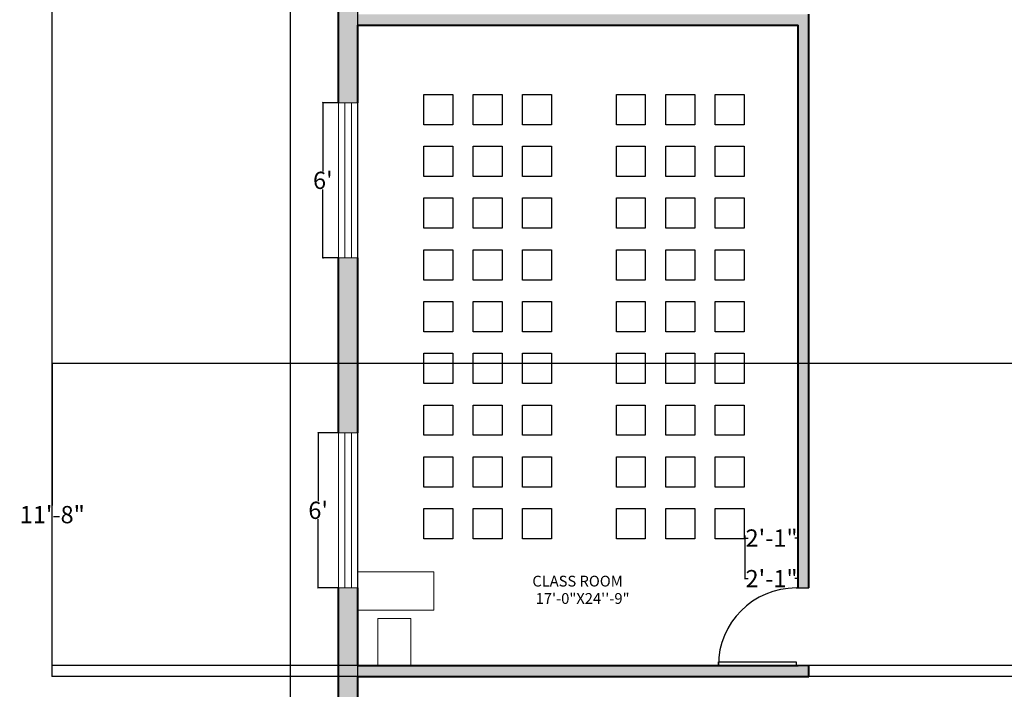
# Model space of a CAD drawing. Units: inches. Extents: x -405 to 940, y 226 to 2032.
# Tile 3 of 10: x -405 to 51, y 846 to 1156. Entities that reach past the tile are written whole.
import ezdxf

# ---------------------------------------------------------------- set-up
doc = ezdxf.new("R2010")
doc.units = ezdxf.units.IN
doc.header["$MEASUREMENT"] = 0
doc.linetypes.add('ACAD_ISO02W100', pattern=[15, 12, -3])
for name, color, linetype, lineweight in [('A-ANNO-DIMS', 120, 'Continuous', 18), ('A-AREA-IDEN', 32, 'Continuous', 18), ('A-FURN-SEAT', 5, 'Continuous', 18), ('A-GLAZ-HIDN', 1, 'ACAD_ISO02W100', 18), ('A-WALL-PATT', 8, 'Continuous', 13), ('door', 6, 'Continuous', 25), ('tables', 2, 'Continuous', 18), ('wall', 3, 'Continuous', 40), ('window', 1, 'Continuous', 18)]:
    doc.layers.add(name, color=color, linetype=linetype, lineweight=lineweight)
doc.layers.add('beches', color=5, linetype='Continuous')
doc.styles.get("Standard").update_dxf_attribs({"font": 'arial.ttf'})
doc.dimstyles.get("Standard").update_dxf_attribs({"dimtxt": 8, "dimasz": 0.18, "dimexe": 0.18, "dimexo": 0.0625, "dimgap": 0.09, "dimtad": 0, "dimtih": 1, "dimtoh": 1, "dimdec": 0, "dimzin": 0, "dimdsep": 46, "dimlunit": 3, "dimtxsty": 'Standard', "dimblk": 'OBLIQUE', "dimcen": 0.09, "dimadec": 0, "dimazin": 0, "dimtfac": 1, "dimtdec": 0, "dimtofl": 0, "dimtmove": 0, "dimatfit": 3, "dimfxl": 1, "dimtolj": 1, "dimtzin": 0, "dimarcsym": 0})

# ---------------------------------------------------------------- blocks, each defined once
blk = doc.blocks.new('*U4')
for p, q in [((0, 0), (0, -6)), ((36, 0), (36, -6))]:
    blk.add_line(p, q)
blk.add_lwpolyline([(0, 0), (0, 36), (1.75, 36), (1.75, 0)], close=True)
blk.add_arc((0, 0), 36, 0, 90)
blk = doc.blocks.new('*U13')
at = {"layer": 'beches'}
blk.add_lwpolyline([(6.71, -7.02), (-6.71, -7.02), (-6.71, 7.02), (6.71, 7.02)], close=True, dxfattribs=at)
blk = doc.blocks.new('*U14')
at = {"layer": 'A-FURN-SEAT', "transparency": 16777216}
for p in [(-45.84, 192), (-45.84, 192, 12), (-45.84, 192, 24), (-45.84, 192, 36), (-45.84, 192, 48), (-45.84, 192, 60), (-45.84, 192, 72), (-45.84, 192, 84), (-45.84, 192, 96), (-45.84, 192, 108), (-45.84, 192, 120), (-45.84, 192, 132), (-22.92, 192), (-22.92, 192, 12), (-22.92, 192, 24), (-22.92, 192, 36), (-22.92, 192, 48), (-22.92, 192, 60), (-22.92, 192, 72), (-22.92, 192, 84), (-22.92, 192, 96), (-22.92, 192, 108), (-22.92, 192, 120), (-22.92, 192, 132), (0, 192), (0, 192, 12), (0, 192, 24), (0, 192, 36), (0, 192, 48), (0, 192, 60), (0, 192, 72), (0, 192, 84), (0, 192, 96), (0, 192, 108), (0, 192, 120), (0, 192, 132), (-45.84, 168), (-45.84, 168, 12), (-45.84, 168, 24), (-45.84, 168, 36), (-45.84, 168, 48), (-45.84, 168, 60), (-45.84, 168, 72), (-45.84, 168, 84), (-45.84, 168, 96), (-45.84, 168, 108), (-45.84, 168, 120), (-45.84, 168, 132), (-22.92, 168), (-22.92, 168, 12), (-22.92, 168, 24), (-22.92, 168, 36), (-22.92, 168, 48), (-22.92, 168, 60), (-22.92, 168, 72), (-22.92, 168, 84), (-22.92, 168, 96), (-22.92, 168, 108), (-22.92, 168, 120), (-22.92, 168, 132), (0, 168), (0, 168, 12), (0, 168, 24), (0, 168, 36), (0, 168, 48), (0, 168, 60), (0, 168, 72), (0, 168, 84), (0, 168, 96), (0, 168, 108), (0, 168, 120), (0, 168, 132), (-45.84, 144), (-45.84, 144, 12), (-45.84, 144, 24), (-45.84, 144, 36), (-45.84, 144, 48), (-45.84, 144, 60), (-45.84, 144, 72), (-45.84, 144, 84), (-45.84, 144, 96), (-45.84, 144, 108), (-45.84, 144, 120), (-45.84, 144, 132), (-22.92, 144), (-22.92, 144, 12), (-22.92, 144, 24), (-22.92, 144, 36), (-22.92, 144, 48), (-22.92, 144, 60), (-22.92, 144, 72), (-22.92, 144, 84), (-22.92, 144, 96), (-22.92, 144, 108), (-22.92, 144, 120), (-22.92, 144, 132), (0, 144), (0, 144, 12), (0, 144, 24), (0, 144, 36), (0, 144, 48), (0, 144, 60), (0, 144, 72), (0, 144, 84), (0, 144, 96), (0, 144, 108), (0, 144, 120), (0, 144, 132), (-45.84, 120), (-45.84, 120, 12), (-45.84, 120, 24), (-45.84, 120, 36), (-45.84, 120, 48), (-45.84, 120, 60), (-45.84, 120, 72), (-45.84, 120, 84), (-45.84, 120, 96), (-45.84, 120, 108), (-45.84, 120, 120), (-45.84, 120, 132), (-22.92, 120), (-22.92, 120, 12), (-22.92, 120, 24), (-22.92, 120, 36), (-22.92, 120, 48), (-22.92, 120, 60), (-22.92, 120, 72), (-22.92, 120, 84), (-22.92, 120, 96), (-22.92, 120, 108), (-22.92, 120, 120), (-22.92, 120, 132), (0, 120), (0, 120, 12), (0, 120, 24), (0, 120, 36), (0, 120, 48), (0, 120, 60), (0, 120, 72), (0, 120, 84), (0, 120, 96), (0, 120, 108), (0, 120, 120), (0, 120, 132), (-45.84, 96), (-45.84, 96, 12), (-45.84, 96, 24), (-45.84, 96, 36), (-45.84, 96, 48), (-45.84, 96, 60), (-45.84, 96, 72), (-45.84, 96, 84), (-45.84, 96, 96), (-45.84, 96, 108), (-45.84, 96, 120), (-45.84, 96, 132), (-22.92, 96), (-22.92, 96, 12), (-22.92, 96, 24), (-22.92, 96, 36), (-22.92, 96, 48), (-22.92, 96, 60), (-22.92, 96, 72), (-22.92, 96, 84), (-22.92, 96, 96), (-22.92, 96, 108), (-22.92, 96, 120), (-22.92, 96, 132), (0, 96), (0, 96, 12), (0, 96, 24), (0, 96, 36), (0, 96, 48), (0, 96, 60), (0, 96, 72), (0, 96, 84), (0, 96, 96), (0, 96, 108), (0, 96, 120), (0, 96, 132), (-45.84, 72), (-45.84, 72, 12), (-45.84, 72, 24), (-45.84, 72, 36), (-45.84, 72, 48), (-45.84, 72, 60), (-45.84, 72, 72), (-45.84, 72, 84), (-45.84, 72, 96), (-45.84, 72, 108), (-45.84, 72, 120), (-45.84, 72, 132), (-22.92, 72), (-22.92, 72, 12), (-22.92, 72, 24), (-22.92, 72, 36), (-22.92, 72, 48), (-22.92, 72, 60), (-22.92, 72, 72), (-22.92, 72, 84), (-22.92, 72, 96), (-22.92, 72, 108), (-22.92, 72, 120), (-22.92, 72, 132), (0, 72), (0, 72, 12), (0, 72, 24), (0, 72, 36), (0, 72, 48), (0, 72, 60), (0, 72, 72), (0, 72, 84), (0, 72, 96), (0, 72, 108), (0, 72, 120), (0, 72, 132), (-45.84, 48), (-45.84, 48, 12), (-45.84, 48, 24), (-45.84, 48, 36), (-45.84, 48, 48), (-45.84, 48, 60), (-45.84, 48, 72), (-45.84, 48, 84), (-45.84, 48, 96), (-45.84, 48, 108), (-45.84, 48, 120), (-45.84, 48, 132), (-22.92, 48), (-22.92, 48, 12), (-22.92, 48, 24), (-22.92, 48, 36), (-22.92, 48, 48), (-22.92, 48, 60), (-22.92, 48, 72), (-22.92, 48, 84), (-22.92, 48, 96), (-22.92, 48, 108), (-22.92, 48, 120), (-22.92, 48, 132), (0, 48), (0, 48, 12), (0, 48, 24), (0, 48, 36), (0, 48, 48), (0, 48, 60), (0, 48, 72), (0, 48, 84), (0, 48, 96), (0, 48, 108), (0, 48, 120), (0, 48, 132), (-45.84, 24), (-45.84, 24, 12), (-45.84, 24, 24), (-45.84, 24, 36), (-45.84, 24, 48), (-45.84, 24, 60), (-45.84, 24, 72), (-45.84, 24, 84), (-45.84, 24, 96), (-45.84, 24, 108), (-45.84, 24, 120), (-45.84, 24, 132), (-22.92, 24), (-22.92, 24, 12), (-22.92, 24, 24), (-22.92, 24, 36), (-22.92, 24, 48), (-22.92, 24, 60), (-22.92, 24, 72), (-22.92, 24, 84), (-22.92, 24, 96), (-22.92, 24, 108), (-22.92, 24, 120), (-22.92, 24, 132), (0, 24), (0, 24, 12), (0, 24, 24), (0, 24, 36), (0, 24, 48), (0, 24, 60), (0, 24, 72), (0, 24, 84), (0, 24, 96), (0, 24, 108), (0, 24, 120), (0, 24, 132), (-45.84, 0), (-45.84, 0, 12), (-45.84, 0, 24), (-45.84, 0, 36), (-45.84, 0, 48), (-45.84, 0, 60), (-45.84, 0, 72), (-45.84, 0, 84), (-45.84, 0, 96), (-45.84, 0, 108), (-45.84, 0, 120), (-45.84, 0, 132), (-22.92, 0), (-22.92, 0, 12), (-22.92, 0, 24), (-22.92, 0, 36), (-22.92, 0, 48), (-22.92, 0, 60), (-22.92, 0, 72), (-22.92, 0, 84), (-22.92, 0, 96), (-22.92, 0, 108), (-22.92, 0, 120), (-22.92, 0, 132), (0, 0), (0, 0, 12), (0, 0, 24), (0, 0, 36), (0, 0, 48), (0, 0, 60), (0, 0, 72), (0, 0, 84), (0, 0, 96), (0, 0, 108), (0, 0, 120), (0, 0, 132)]:
    blk.add_blockref('*U13', p, dxfattribs=at)
blk = doc.blocks.new('*U11')
at = {"layer": 'beches'}
blk.add_lwpolyline([(6.71, -7.02), (-6.71, -7.02), (-6.71, 7.02), (6.71, 7.02)], close=True, dxfattribs=at)
blk = doc.blocks.new('*U12')
at = {"layer": 'A-FURN-SEAT', "transparency": 16777216}
for p in [(-45.84, 192), (-45.84, 192, 12), (-45.84, 192, 24), (-45.84, 192, 36), (-45.84, 192, 48), (-45.84, 192, 60), (-45.84, 192, 72), (-45.84, 192, 84), (-45.84, 192, 96), (-45.84, 192, 108), (-45.84, 192, 120), (-45.84, 192, 132), (-22.92, 192), (-22.92, 192, 12), (-22.92, 192, 24), (-22.92, 192, 36), (-22.92, 192, 48), (-22.92, 192, 60), (-22.92, 192, 72), (-22.92, 192, 84), (-22.92, 192, 96), (-22.92, 192, 108), (-22.92, 192, 120), (-22.92, 192, 132), (0, 192), (0, 192, 12), (0, 192, 24), (0, 192, 36), (0, 192, 48), (0, 192, 60), (0, 192, 72), (0, 192, 84), (0, 192, 96), (0, 192, 108), (0, 192, 120), (0, 192, 132), (-45.84, 168), (-45.84, 168, 12), (-45.84, 168, 24), (-45.84, 168, 36), (-45.84, 168, 48), (-45.84, 168, 60), (-45.84, 168, 72), (-45.84, 168, 84), (-45.84, 168, 96), (-45.84, 168, 108), (-45.84, 168, 120), (-45.84, 168, 132), (-22.92, 168), (-22.92, 168, 12), (-22.92, 168, 24), (-22.92, 168, 36), (-22.92, 168, 48), (-22.92, 168, 60), (-22.92, 168, 72), (-22.92, 168, 84), (-22.92, 168, 96), (-22.92, 168, 108), (-22.92, 168, 120), (-22.92, 168, 132), (0, 168), (0, 168, 12), (0, 168, 24), (0, 168, 36), (0, 168, 48), (0, 168, 60), (0, 168, 72), (0, 168, 84), (0, 168, 96), (0, 168, 108), (0, 168, 120), (0, 168, 132), (-45.84, 144), (-45.84, 144, 12), (-45.84, 144, 24), (-45.84, 144, 36), (-45.84, 144, 48), (-45.84, 144, 60), (-45.84, 144, 72), (-45.84, 144, 84), (-45.84, 144, 96), (-45.84, 144, 108), (-45.84, 144, 120), (-45.84, 144, 132), (-22.92, 144), (-22.92, 144, 12), (-22.92, 144, 24), (-22.92, 144, 36), (-22.92, 144, 48), (-22.92, 144, 60), (-22.92, 144, 72), (-22.92, 144, 84), (-22.92, 144, 96), (-22.92, 144, 108), (-22.92, 144, 120), (-22.92, 144, 132), (0, 144), (0, 144, 12), (0, 144, 24), (0, 144, 36), (0, 144, 48), (0, 144, 60), (0, 144, 72), (0, 144, 84), (0, 144, 96), (0, 144, 108), (0, 144, 120), (0, 144, 132), (-45.84, 120), (-45.84, 120, 12), (-45.84, 120, 24), (-45.84, 120, 36), (-45.84, 120, 48), (-45.84, 120, 60), (-45.84, 120, 72), (-45.84, 120, 84), (-45.84, 120, 96), (-45.84, 120, 108), (-45.84, 120, 120), (-45.84, 120, 132), (-22.92, 120), (-22.92, 120, 12), (-22.92, 120, 24), (-22.92, 120, 36), (-22.92, 120, 48), (-22.92, 120, 60), (-22.92, 120, 72), (-22.92, 120, 84), (-22.92, 120, 96), (-22.92, 120, 108), (-22.92, 120, 120), (-22.92, 120, 132), (0, 120), (0, 120, 12), (0, 120, 24), (0, 120, 36), (0, 120, 48), (0, 120, 60), (0, 120, 72), (0, 120, 84), (0, 120, 96), (0, 120, 108), (0, 120, 120), (0, 120, 132), (-45.84, 96), (-45.84, 96, 12), (-45.84, 96, 24), (-45.84, 96, 36), (-45.84, 96, 48), (-45.84, 96, 60), (-45.84, 96, 72), (-45.84, 96, 84), (-45.84, 96, 96), (-45.84, 96, 108), (-45.84, 96, 120), (-45.84, 96, 132), (-22.92, 96), (-22.92, 96, 12), (-22.92, 96, 24), (-22.92, 96, 36), (-22.92, 96, 48), (-22.92, 96, 60), (-22.92, 96, 72), (-22.92, 96, 84), (-22.92, 96, 96), (-22.92, 96, 108), (-22.92, 96, 120), (-22.92, 96, 132), (0, 96), (0, 96, 12), (0, 96, 24), (0, 96, 36), (0, 96, 48), (0, 96, 60), (0, 96, 72), (0, 96, 84), (0, 96, 96), (0, 96, 108), (0, 96, 120), (0, 96, 132), (-45.84, 72), (-45.84, 72, 12), (-45.84, 72, 24), (-45.84, 72, 36), (-45.84, 72, 48), (-45.84, 72, 60), (-45.84, 72, 72), (-45.84, 72, 84), (-45.84, 72, 96), (-45.84, 72, 108), (-45.84, 72, 120), (-45.84, 72, 132), (-22.92, 72), (-22.92, 72, 12), (-22.92, 72, 24), (-22.92, 72, 36), (-22.92, 72, 48), (-22.92, 72, 60), (-22.92, 72, 72), (-22.92, 72, 84), (-22.92, 72, 96), (-22.92, 72, 108), (-22.92, 72, 120), (-22.92, 72, 132), (0, 72), (0, 72, 12), (0, 72, 24), (0, 72, 36), (0, 72, 48), (0, 72, 60), (0, 72, 72), (0, 72, 84), (0, 72, 96), (0, 72, 108), (0, 72, 120), (0, 72, 132), (-45.84, 48), (-45.84, 48, 12), (-45.84, 48, 24), (-45.84, 48, 36), (-45.84, 48, 48), (-45.84, 48, 60), (-45.84, 48, 72), (-45.84, 48, 84), (-45.84, 48, 96), (-45.84, 48, 108), (-45.84, 48, 120), (-45.84, 48, 132), (-22.92, 48), (-22.92, 48, 12), (-22.92, 48, 24), (-22.92, 48, 36), (-22.92, 48, 48), (-22.92, 48, 60), (-22.92, 48, 72), (-22.92, 48, 84), (-22.92, 48, 96), (-22.92, 48, 108), (-22.92, 48, 120), (-22.92, 48, 132), (0, 48), (0, 48, 12), (0, 48, 24), (0, 48, 36), (0, 48, 48), (0, 48, 60), (0, 48, 72), (0, 48, 84), (0, 48, 96), (0, 48, 108), (0, 48, 120), (0, 48, 132), (-45.84, 24), (-45.84, 24, 12), (-45.84, 24, 24), (-45.84, 24, 36), (-45.84, 24, 48), (-45.84, 24, 60), (-45.84, 24, 72), (-45.84, 24, 84), (-45.84, 24, 96), (-45.84, 24, 108), (-45.84, 24, 120), (-45.84, 24, 132), (-22.92, 24), (-22.92, 24, 12), (-22.92, 24, 24), (-22.92, 24, 36), (-22.92, 24, 48), (-22.92, 24, 60), (-22.92, 24, 72), (-22.92, 24, 84), (-22.92, 24, 96), (-22.92, 24, 108), (-22.92, 24, 120), (-22.92, 24, 132), (0, 24), (0, 24, 12), (0, 24, 24), (0, 24, 36), (0, 24, 48), (0, 24, 60), (0, 24, 72), (0, 24, 84), (0, 24, 96), (0, 24, 108), (0, 24, 120), (0, 24, 132), (-45.84, 0), (-45.84, 0, 12), (-45.84, 0, 24), (-45.84, 0, 36), (-45.84, 0, 48), (-45.84, 0, 60), (-45.84, 0, 72), (-45.84, 0, 84), (-45.84, 0, 96), (-45.84, 0, 108), (-45.84, 0, 120), (-45.84, 0, 132), (-22.92, 0), (-22.92, 0, 12), (-22.92, 0, 24), (-22.92, 0, 36), (-22.92, 0, 48), (-22.92, 0, 60), (-22.92, 0, 72), (-22.92, 0, 84), (-22.92, 0, 96), (-22.92, 0, 108), (-22.92, 0, 120), (-22.92, 0, 132), (0, 0), (0, 0, 12), (0, 0, 24), (0, 0, 36), (0, 0, 48), (0, 0, 60), (0, 0, 72), (0, 0, 84), (0, 0, 96), (0, 0, 108), (0, 0, 120), (0, 0, 132)]:
    blk.add_blockref('*U11', p, dxfattribs=at)
blk = doc.blocks.new('_Oblique')
at = {"color": 0, "linetype": 'ByBlock', "lineweight": -2}
blk.add_line((-0.5, -0.5), (0.5, 0.5), dxfattribs=at)
blk = doc.blocks.new('*D44')
at = {"layer": 'A-ANNO-DIMS', "color": 0, "lineweight": -2, "transparency": 16777216}
for p, q in [((-257.29, 1887.81), (-279.61, 1887.81)), ((-279.43, 1887.81), (-279.43, 1210.99)), ((-279.43, 525.81), (-279.43, 1202.63)), ((-257.29, 525.81), (-279.61, 525.81))]:
    blk.add_line(p, q, dxfattribs=at)
at = {"layer": 'Defpoints', "color": 0, "transparency": 16777216}
for p in [(-257.23, 1887.81), (-279.43, 525.81), (-257.23, 525.81)]:
    blk.add_point(p, dxfattribs=at)
at = {"layer": 'A-ANNO-DIMS', "color": 0, "lineweight": -2, "transparency": 16777216, "xscale": 0.18, "yscale": 0.18, "zscale": 0.18}
for p, rotation in [((-279.43, 1887.81), 90), ((-279.43, 525.81), 270)]:
    blk.add_blockref('_Oblique', p, dxfattribs=dict(at, rotation=rotation))
at = {"layer": 'A-ANNO-DIMS', "color": 0, "transparency": 16777216, "insert": (-279.43, 1206.81), "char_height": 8, "attachment_point": 5}
blk.add_mtext('\\A1;113\'-6"', dxfattribs=at)
blk = doc.blocks.new('*D45')
at = {"layer": 'A-ANNO-DIMS', "color": 0, "lineweight": -2, "transparency": 16777216}
for p, q in [((-68.93, 917.09), (-68.93, 915.78)), ((-44.23, 917.09), (-44.23, 915.78)), ((-68.93, 915.96), (-67.37, 915.96)), ((-44.23, 915.96), (-45.79, 915.96))]:
    blk.add_line(p, q, dxfattribs=at)
at = {"layer": 'Defpoints', "color": 0, "transparency": 16777216}
for p in [(-68.93, 917.16), (-44.23, 917.16), (-68.93, 915.96)]:
    blk.add_point(p, dxfattribs=at)
at = {"layer": 'A-ANNO-DIMS', "color": 0, "lineweight": -2, "transparency": 16777216, "xscale": 0.18, "yscale": 0.18, "zscale": 0.18, "rotation": 180}
blk.add_blockref('_Oblique', (-68.93, 915.96), dxfattribs=at)
at = {"layer": 'A-ANNO-DIMS', "color": 0, "lineweight": -2, "transparency": 16777216, "xscale": 0.18, "yscale": 0.18, "zscale": 0.18}
blk.add_blockref('_Oblique', (-44.23, 915.96), dxfattribs=at)
at = {"layer": 'A-ANNO-DIMS', "color": 0, "transparency": 16777216, "insert": (-56.58, 915.96), "char_height": 8, "attachment_point": 5}
blk.add_mtext('\\A1;2\'-1"', dxfattribs=at)
blk = doc.blocks.new('*D46')
at = {"layer": 'A-ANNO-DIMS', "color": 0, "lineweight": -2, "transparency": 16777216}
for p, q in [((-68.93, 915.72), (-68.93, 896.95)), ((-68.93, 897.13), (-67.37, 897.13)), ((-44.23, 897.13), (-45.79, 897.13)), ((-44.23, 892.87), (-44.23, 897.31))]:
    blk.add_line(p, q, dxfattribs=at)
at = {"layer": 'Defpoints', "color": 0, "transparency": 16777216}
for p in [(-68.93, 915.78), (-44.23, 897.13), (-44.23, 892.81)]:
    blk.add_point(p, dxfattribs=at)
at = {"layer": 'A-ANNO-DIMS', "color": 0, "lineweight": -2, "transparency": 16777216, "xscale": 0.18, "yscale": 0.18, "zscale": 0.18, "rotation": 180}
blk.add_blockref('_Oblique', (-68.93, 897.13), dxfattribs=at)
at = {"layer": 'A-ANNO-DIMS', "color": 0, "lineweight": -2, "transparency": 16777216, "xscale": 0.18, "yscale": 0.18, "zscale": 0.18}
blk.add_blockref('_Oblique', (-44.23, 897.13), dxfattribs=at)
at = {"layer": 'A-ANNO-DIMS', "color": 0, "transparency": 16777216, "insert": (-56.58, 897.13), "char_height": 8, "attachment_point": 5}
blk.add_mtext('\\A1;2\'-1"', dxfattribs=at)
blk = doc.blocks.new('*D53')
at = {"layer": 'A-ANNO-DIMS', "color": 0, "lineweight": -2, "transparency": 16777216}
for p, q in [((-257.29, 964.81), (-266.86, 964.81)), ((-266.68, 964.81), (-266.68, 932.98)), ((-266.68, 892.81), (-266.68, 924.64)), ((-257.29, 892.81), (-266.86, 892.81))]:
    blk.add_line(p, q, dxfattribs=at)
at = {"layer": 'Defpoints', "color": 0, "transparency": 16777216}
for p in [(-266.68, 964.81), (-257.23, 964.81), (-257.23, 892.81)]:
    blk.add_point(p, dxfattribs=at)
at = {"layer": 'A-ANNO-DIMS', "color": 0, "lineweight": -2, "transparency": 16777216, "xscale": 0.18, "yscale": 0.18, "zscale": 0.18}
for p, rotation in [((-266.68, 964.81), 90), ((-266.68, 892.81), 270)]:
    blk.add_blockref('_Oblique', p, dxfattribs=dict(at, rotation=rotation))
at = {"layer": 'A-ANNO-DIMS', "color": 0, "transparency": 16777216, "insert": (-266.68, 928.81), "char_height": 8, "attachment_point": 5}
blk.add_mtext("\\A1;6'", dxfattribs=at)
blk = doc.blocks.new('*D54')
at = {"layer": 'A-ANNO-DIMS', "color": 0, "lineweight": -2, "transparency": 16777216}
for p, q in [((-257.29, 1117.81), (-264.68, 1117.81)), ((-264.5, 1117.81), (-264.5, 1085.98)), ((-264.5, 1045.81), (-264.5, 1077.64)), ((-257.29, 1045.81), (-264.68, 1045.81))]:
    blk.add_line(p, q, dxfattribs=at)
at = {"layer": 'Defpoints', "color": 0, "transparency": 16777216}
for p in [(-264.5, 1117.81), (-257.23, 1117.81), (-257.23, 1045.81)]:
    blk.add_point(p, dxfattribs=at)
at = {"layer": 'A-ANNO-DIMS', "color": 0, "lineweight": -2, "transparency": 16777216, "xscale": 0.18, "yscale": 0.18, "zscale": 0.18}
for p, rotation in [((-264.5, 1117.81), 90), ((-264.5, 1045.81), 270)]:
    blk.add_blockref('_Oblique', p, dxfattribs=dict(at, rotation=rotation))
at = {"layer": 'A-ANNO-DIMS', "color": 0, "transparency": 16777216, "insert": (-264.5, 1081.81), "char_height": 8, "attachment_point": 5}
blk.add_mtext("\\A1;6'", dxfattribs=at)
blk = doc.blocks.new('WIN-PANE-72IN')
for p, q in [((0, 3), (72, 3)), ((0, 0), (72, 0))]:
    blk.add_line(p, q)
blk = doc.blocks.new('*D107')
at = {"layer": 'A-ANNO-DIMS', "color": 0, "lineweight": -2, "transparency": 16777216}
for p, q in [((501.71, 1597.81), (-390.06, 1597.81)), ((-389.88, 1597.81), (-389.88, 1228.98)), ((-389.88, 851.81), (-389.88, 1220.64)), ((501.71, 851.81), (-390.06, 851.81))]:
    blk.add_line(p, q, dxfattribs=at)
at = {"layer": 'Defpoints', "color": 0, "transparency": 16777216}
for p in [(-389.88, 1597.81), (501.77, 1597.81), (501.77, 851.81)]:
    blk.add_point(p, dxfattribs=at)
at = {"layer": 'A-ANNO-DIMS', "color": 0, "lineweight": -2, "transparency": 16777216, "xscale": 0.18, "yscale": 0.18, "zscale": 0.18}
for p, rotation in [((-389.88, 1597.81), 90), ((-389.88, 851.81), 270)]:
    blk.add_blockref('_Oblique', p, dxfattribs=dict(at, rotation=rotation))
at = {"layer": 'A-ANNO-DIMS', "color": 0, "transparency": 16777216, "insert": (-389.88, 1224.81), "char_height": 8, "attachment_point": 5}
blk.add_mtext('\\A1;62\'-2"', dxfattribs=at)
blk = doc.blocks.new('*D108')
at = {"layer": 'A-ANNO-DIMS', "color": 0, "lineweight": -2, "transparency": 16777216}
for p, q in [((806.71, 996.81), (-390.06, 996.81)), ((-389.88, 996.81), (-389.88, 930.98)), ((-389.88, 856.81), (-389.88, 922.64)), ((806.71, 856.81), (-390.06, 856.81))]:
    blk.add_line(p, q, dxfattribs=at)
at = {"layer": 'Defpoints', "color": 0, "transparency": 16777216}
for p in [(-389.88, 996.81), (806.77, 996.81), (806.77, 856.81)]:
    blk.add_point(p, dxfattribs=at)
at = {"layer": 'A-ANNO-DIMS', "color": 0, "lineweight": -2, "transparency": 16777216, "xscale": 0.18, "yscale": 0.18, "zscale": 0.18}
for p, rotation in [((-389.88, 996.81), 90), ((-389.88, 856.81), 270)]:
    blk.add_blockref('_Oblique', p, dxfattribs=dict(at, rotation=rotation))
at = {"layer": 'A-ANNO-DIMS', "color": 0, "transparency": 16777216, "insert": (-389.88, 926.81), "char_height": 8, "attachment_point": 5}
blk.add_mtext('\\A1;11\'-8"', dxfattribs=at)
blk = doc.blocks.new('*D109')
at = {"layer": 'A-ANNO-DIMS', "color": 0, "lineweight": -2, "transparency": 16777216}
for p, q in [((-248.23, 750.87), (-248.23, 2020.64)), ((-248.23, 2020.46), (-49.06, 2020.46)), ((177.77, 2020.46), (-21.4, 2020.46)), ((177.77, 750.87), (177.77, 2020.64))]:
    blk.add_line(p, q, dxfattribs=at)
at = {"layer": 'Defpoints', "color": 0, "transparency": 16777216}
for p in [(177.77, 2020.46), (-248.23, 750.81), (177.77, 750.81)]:
    blk.add_point(p, dxfattribs=at)
at = {"layer": 'A-ANNO-DIMS', "color": 0, "lineweight": -2, "transparency": 16777216, "xscale": 0.18, "yscale": 0.18, "zscale": 0.18, "rotation": 180}
blk.add_blockref('_Oblique', (-248.23, 2020.46), dxfattribs=at)
at = {"layer": 'A-ANNO-DIMS', "color": 0, "lineweight": -2, "transparency": 16777216, "xscale": 0.18, "yscale": 0.18, "zscale": 0.18}
blk.add_blockref('_Oblique', (177.77, 2020.46), dxfattribs=at)
at = {"layer": 'A-ANNO-DIMS', "color": 0, "transparency": 16777216, "insert": (-35.23, 2020.46), "char_height": 8, "attachment_point": 5}
blk.add_mtext('\\A1;35\'-6"', dxfattribs=at)

msp = doc.modelspace()

# ---------------------------------------------------------------- hatches: boundary and pattern name
at = {"layer": 'A-WALL-PATT'}
h = msp.add_hatch(dxfattribs=at)
h.set_pattern_fill('AR-HBONE', color=256)
h.set_pattern_definition([(45, (599.8442, 904.9158), (0, 5.656854), [12, -4]), (135, (602.6726, 907.744), (4e-16, 5.656854), [12, -4])])
h.paths.add_polyline_path([(-248.23, 1045.81), (-257.23, 1045.81), (-257.23, 964.81), (-248.23, 964.81)], flags=17)
h.paths.add_polyline_path([(-248.23, 851.81), (-39.23, 851.81), (-39.23, 856.81), (-44.23, 856.81), (-248.23, 856.81), (-248.23, 892.81), (-257.23, 892.81), (-257.23, 839.81), (-248.23, 839.81)])
h.paths.add_polyline_path([(-248.23, 750.81), (124.74, 750.81), (124.74, 751.73), (124.74, 755.81), (-248.23, 755.81), (-248.23, 767.81), (-257.23, 767.81), (-257.23, 726.81), (-248.23, 726.81)])
h.paths.add_polyline_path([(-248.23, 654.81), (-257.23, 654.81), (-257.23, 630.81), (-248.23, 630.81)])
h.paths.add_polyline_path([(-180.23, 534.81), (-248.23, 534.81), (-248.23, 558.81), (-257.23, 558.81), (-257.23, 525.81), (-180.23, 525.81)])
h.paths.add_polyline_path([(-69.23, 534.81), (-108.23, 534.81), (-108.23, 525.81), (-69.23, 525.81)])
h.paths.add_polyline_path([(35.77, 534.81), (2.77, 534.81), (2.77, 525.81), (35.77, 525.81)])
h.paths.add_polyline_path([(182.77, 755.81), (160.74, 755.81), (160.74, 750.81), (177.77, 750.81), (177.77, 534.81), (107.77, 534.81), (107.77, 525.81), (182.77, 525.81)])
h.paths.add_polyline_path([(-39.23, 1609.81), (-44.23, 1609.81), (-44.23, 1604.81), (-44.23, 1460.81), (-135.23, 1460.81), (-135.23, 1465.73), (-140.23, 1465.73), (-140.23, 1460.81), (-248.23, 1460.81), (-248.23, 1471.31), (-257.23, 1471.31), (-257.23, 1419.81), (-248.23, 1419.81), (-248.23, 1455.81), (-44.23, 1455.81), (-44.23, 1194.81), (-39.23, 1194.81)])
h.paths.add_polyline_path([(-248.23, 1520.81), (-257.23, 1520.81), (-257.23, 1495.31), (-248.23, 1495.31), (-248.23, 1505.81), (-140.23, 1505.81), (-140.23, 1495.73), (-135.23, 1495.73), (-135.23, 1516.79), (-140.23, 1516.79), (-140.23, 1510.81), (-248.23, 1510.81)], flags=17)
h.paths.add_polyline_path([(-248.23, 1570.31), (-257.23, 1570.31), (-257.23, 1544.81), (-248.23, 1544.81), (-248.23, 1554.81), (-140.23, 1554.81), (-140.23, 1546.79), (-135.23, 1546.79), (-135.23, 1565.08), (-140.23, 1565.08), (-140.23, 1559.81), (-248.23, 1559.81)], flags=17)
h.paths.add_polyline_path([(-248.23, 1615.81), (-257.23, 1615.81), (-257.23, 1594.31), (-248.23, 1594.31), (-248.23, 1604.81), (-140.23, 1604.81), (-140.23, 1595.08), (-135.23, 1595.08), (-135.23, 1604.81), (-80.23, 1604.81), (-80.23, 1609.81), (-248.23, 1609.81)])
h.paths.add_polyline_path([(-248.23, 1783.81), (-235.46, 1783.81), (-235.46, 1788.81), (-248.23, 1788.81), (-248.23, 1878.81), (-237.73, 1878.81), (-237.73, 1887.81), (-257.23, 1887.81), (-257.23, 1687.81), (-248.23, 1687.81), (-248.23, 1693.81), (-136.23, 1693.81), (-136.23, 1698.81), (-248.23, 1698.81)])
h.paths.add_polyline_path([(-188.23, 1887.81), (-213.73, 1887.81), (-213.73, 1878.81), (-203.23, 1878.81), (-203.23, 1788.81), (-205.46, 1788.81), (-205.46, 1783.81), (-186.39, 1783.81), (-186.39, 1788.81), (-198.23, 1788.81), (-198.23, 1878.81), (-188.23, 1878.81)])
h.paths.add_polyline_path([(-139.23, 1887.81), (-164.23, 1887.81), (-164.23, 1878.81), (-154.23, 1878.81), (-154.23, 1788.81), (-156.39, 1788.81), (-156.39, 1783.81), (-138.25, 1783.81), (-138.25, 1788.81), (-149.23, 1788.81), (-149.23, 1878.81), (-139.23, 1878.81)])
h.paths.add_polyline_path([(-89.23, 1887.81), (-115.23, 1887.81), (-115.23, 1878.81), (-105.23, 1878.81), (-105.23, 1788.81), (-108.25, 1788.81), (-108.25, 1783.81), (-86.45, 1783.81), (-86.45, 1788.81), (-100.23, 1788.81), (-100.23, 1878.81), (-89.23, 1878.81)])
h.paths.add_polyline_path([(-36.23, 1887.81), (-65.23, 1887.81), (-65.23, 1878.81), (-54.23, 1878.81), (-54.23, 1788.81), (-56.45, 1788.81), (-56.45, 1783.81), (-54.23, 1783.81), (-54.23, 1698.81), (-100.23, 1698.81), (-100.23, 1693.81), (-49.23, 1693.81), (-49.23, 1698.81), (-49.23, 1878.81), (-36.23, 1878.81)])
h.paths.add_polyline_path([(89.77, 1887.81), (35.77, 1887.81), (35.77, 1878.81), (48.77, 1878.81), (48.77, 1698.81), (-13.23, 1698.81), (-13.23, 1693.81), (53.77, 1693.81), (53.77, 1698.81), (53.77, 1878.81), (89.77, 1878.81)])
h.paths.add_polyline_path([(255.27, 1887.81), (161.77, 1887.81), (161.77, 1878.81), (197.77, 1878.81), (197.77, 1698.81), (89.77, 1698.81), (89.77, 1693.81), (202.77, 1693.81), (202.77, 1698.81), (202.77, 1878.81), (255.27, 1878.81)])
h.paths.add_polyline_path([(375.27, 1887.81), (327.27, 1887.81), (327.27, 1878.81), (375.27, 1878.81)], flags=17)
h.paths.add_polyline_path([(815.77, 1887.81), (447.27, 1887.81), (447.27, 1878.81), (499.77, 1878.81), (499.77, 1698.81), (238.77, 1698.81), (238.77, 1693.81), (504.77, 1693.81), (504.77, 1878.81), (633.77, 1878.81), (633.77, 1646.81), (597.77, 1646.81), (597.77, 1641.81), (602.77, 1641.81), (638.77, 1641.81), (638.77, 1878.81), (806.77, 1878.81), (806.77, 1838.31), (815.77, 1838.31)])
h.paths.add_polyline_path([(815.77, 1766.31), (806.77, 1766.31), (806.77, 1718.31), (815.77, 1718.31)], flags=17)
h.paths.add_polyline_path([(815.77, 1356.31), (806.77, 1356.31), (806.77, 1303.81), (602.77, 1303.81), (597.77, 1303.81), (597.77, 1037.81), (602.77, 1037.81), (602.77, 1298.81), (806.77, 1298.81), (806.77, 1246.31), (815.77, 1246.31)])
h.paths.add_polyline_path([(815.77, 1174.31), (806.77, 1174.31), (806.77, 1126.31), (815.77, 1126.31)], flags=17)
h.paths.add_polyline_path([(815.77, 1054.31), (806.77, 1054.31), (806.77, 1001.81), (796.08, 1001.81), (796.08, 1001.75), (780.86, 1001.75), (602.77, 1001.81), (597.77, 1001.81), (597.77, 892.81), (602.77, 892.81), (602.77, 996.81), (806.77, 996.81), (806.77, 962.81), (815.77, 962.81)])
h.paths.add_polyline_path([(403.77, 534.81), (379.77, 534.81), (379.77, 525.81), (403.77, 525.81)])
h.paths.add_polyline_path([(-39.23, 1158.81), (-44.23, 1158.81), (-248.23, 1158.81), (-248.23, 1194.81), (-257.23, 1194.81), (-257.23, 1117.81), (-248.23, 1117.81), (-248.23, 1153.81), (-44.23, 1153.81), (-44.23, 892.81), (-39.23, 892.81)])
h.paths.add_polyline_path([(-248.23, 1347.81), (-257.23, 1347.81), (-257.23, 1275.81), (-248.23, 1275.81)], flags=17)
h.paths.add_polyline_path([(815.77, 1476.31), (806.77, 1476.31), (806.77, 1428.31), (815.77, 1428.31)], flags=17)
h.paths.add_polyline_path([(815.77, 1646.31), (806.77, 1646.31), (806.77, 1638.65), (806.77, 1605.81), (597.77, 1605.81), (597.77, 1339.81), (602.77, 1339.81), (602.77, 1600.81), (806.77, 1600.81), (806.77, 1548.31), (815.77, 1548.31)])

# ---------------------------------------------------------------- linework, layer by layer
at = {"layer": 'A-FURN-SEAT'}
msp.add_lwpolyline([(-239, 856.81), (-239, 878.62), (-223.78, 878.62), (-223.78, 856.81)], close=True, dxfattribs=at)
at = {"layer": 'A-GLAZ-HIDN'}
for p, q in [((-248.23, 1117.81), (-257.23, 1117.81)), ((-248.23, 1045.81), (-257.23, 1045.81)), ((-248.23, 964.81), (-257.23, 964.81)), ((-248.23, 892.81), (-257.23, 892.81))]:
    msp.add_line(p, q, dxfattribs=at)
at = {"layer": 'door'}
for p, q in [((-44.23, 892.81), (-39.23, 892.81)), ((-44.23, 856.81), (-39.23, 856.81))]:
    msp.add_line(p, q, dxfattribs=at)
at = {"layer": 'tables'}
for p, q in [((-248.23, 882.5), (-248.23, 900.25)), ((-213.09, 900.25), (-248.23, 900.25)), ((-213.09, 900.25), (-213.09, 882.5)), ((-213.09, 882.5), (-248.23, 882.5))]:
    msp.add_line(p, q, dxfattribs=at)
at = {"layer": 'wall'}
for p, q in [((-257.23, 1117.81), (-257.23, 1194.81)), ((-39.23, 892.81), (-39.23, 1158.81)), ((-248.23, 1153.81), (-44.23, 1153.81)), ((-248.23, 1117.81), (-248.23, 1153.81)), ((-44.23, 892.81), (-44.23, 1153.81)), ((-257.23, 964.81), (-257.23, 1045.81)), ((-248.23, 964.81), (-248.23, 1045.81)), ((-257.23, 839.81), (-257.23, 892.81)), ((-248.23, 856.81), (-248.23, 892.81)), ((-248.23, 856.81), (-44.23, 856.81)), ((-39.23, 851.81), (-39.23, 856.81)), ((-248.23, 851.81), (-39.23, 851.81)), ((-248.23, 839.81), (-248.23, 851.81))]:
    msp.add_line(p, q, dxfattribs=at)
at = {"layer": 'window'}
for p, q in [((-257.23, 1045.81), (-257.23, 1117.81)), ((-248.23, 1045.81), (-248.23, 1117.81)), ((-257.23, 892.81), (-257.23, 964.81)), ((-248.23, 892.81), (-248.23, 964.81))]:
    msp.add_line(p, q, dxfattribs=at)

# ---------------------------------------------------------------- block references
at = {"layer": 'A-FURN-SEAT'}
for name, p in [('*U12', (-165.21, 922.62)), ('*U14', (-75.94, 922.62))]:
    msp.add_blockref(name, p, dxfattribs=at)
at = {"layer": 'door', "rotation": 90}
msp.add_blockref('*U4', (-45.23, 856.81), dxfattribs=at)
at = {"layer": 'window'}
for p, rotation in [((-251.23, 1045.81), 90.0000000000001), ((-251.23, 892.81), 90.00000000000003)]:
    msp.add_blockref('WIN-PANE-72IN', p, dxfattribs=dict(at, rotation=rotation))

# ---------------------------------------------------------------- texts
at = {"layer": 'A-AREA-IDEN'}
for s, p in [('CLASS ROOM ', (-167.42, 893.47)), (' 17\'-0"X24\'\'-9"', (-167.42, 885.43))]:
    msp.add_text(s, height=5, dxfattribs=at).set_placement(p)

# ---------------------------------------------------------------- dimensions: what is measured, and where the dimension line sits
at = {"layer": 'A-ANNO-DIMS'}
for base, p1, p2, override, picture, middle in [((177.77, 2020.46), (-248.23, 750.81), (177.77, 750.81), {"dimdec": 1, "dimlfac": 1, "dimrnd": 0, "dimzin": 1, "dimdsep": 46, "dimlunit": 4, "dimfrac": 2}, '*D109', (-35.23, 2020.46)), ((-68.93, 915.96), (-44.23, 917.16), (-68.93, 917.16), {"dimclrd": 0, "dimclre": 0, "dimclrt": 0}, '*D45', (-56.58, 915.96)), ((-44.23, 897.13), (-68.93, 915.78), (-44.23, 892.81), {"dimclrd": 0, "dimclre": 0, "dimclrt": 0}, '*D46', (-56.58, 897.13))]:
    dim = msp.add_linear_dim(base=base, p1=p1, p2=p2, dimstyle='Standard', override=override, dxfattribs=at)
    dim.commit()
    dim.dimension.update_dxf_attribs({"geometry": picture, "text_midpoint": middle})
for base, p1, p2, override, picture, middle in [((-279.43, 525.81), (-257.23, 1887.81), (-257.23, 525.81), {"dimclrd": 0, "dimclre": 0, "dimclrt": 0}, '*D44', (-279.43, 1206.81)), ((-389.88, 1597.81), (501.77, 851.81), (501.77, 1597.81), {"dimdec": 1, "dimlfac": 1, "dimrnd": 0, "dimzin": 1, "dimdsep": 46, "dimlunit": 4, "dimfrac": 2}, '*D107', (-389.88, 1224.81)), ((-264.5, 1117.81), (-257.23, 1045.81), (-257.23, 1117.81), {"dimclrd": 0, "dimclre": 0, "dimclrt": 0}, '*D54', (-264.5, 1081.81)), ((-389.88, 996.81), (806.77, 856.81), (806.77, 996.81), {"dimdec": 1, "dimlfac": 1, "dimrnd": 0, "dimzin": 1, "dimdsep": 46, "dimlunit": 4, "dimfrac": 2}, '*D108', (-389.88, 926.81)), ((-266.68, 964.81), (-257.23, 892.81), (-257.23, 964.81), {"dimclrd": 0, "dimclre": 0, "dimclrt": 0}, '*D53', (-266.68, 928.81))]:
    dim = msp.add_linear_dim(base=base, p1=p1, p2=p2, angle=90, dimstyle='Standard', override=override, dxfattribs=at)
    dim.commit()
    dim.dimension.update_dxf_attribs({"geometry": picture, "text_midpoint": middle})

doc.saveas('drawing.dxf')
